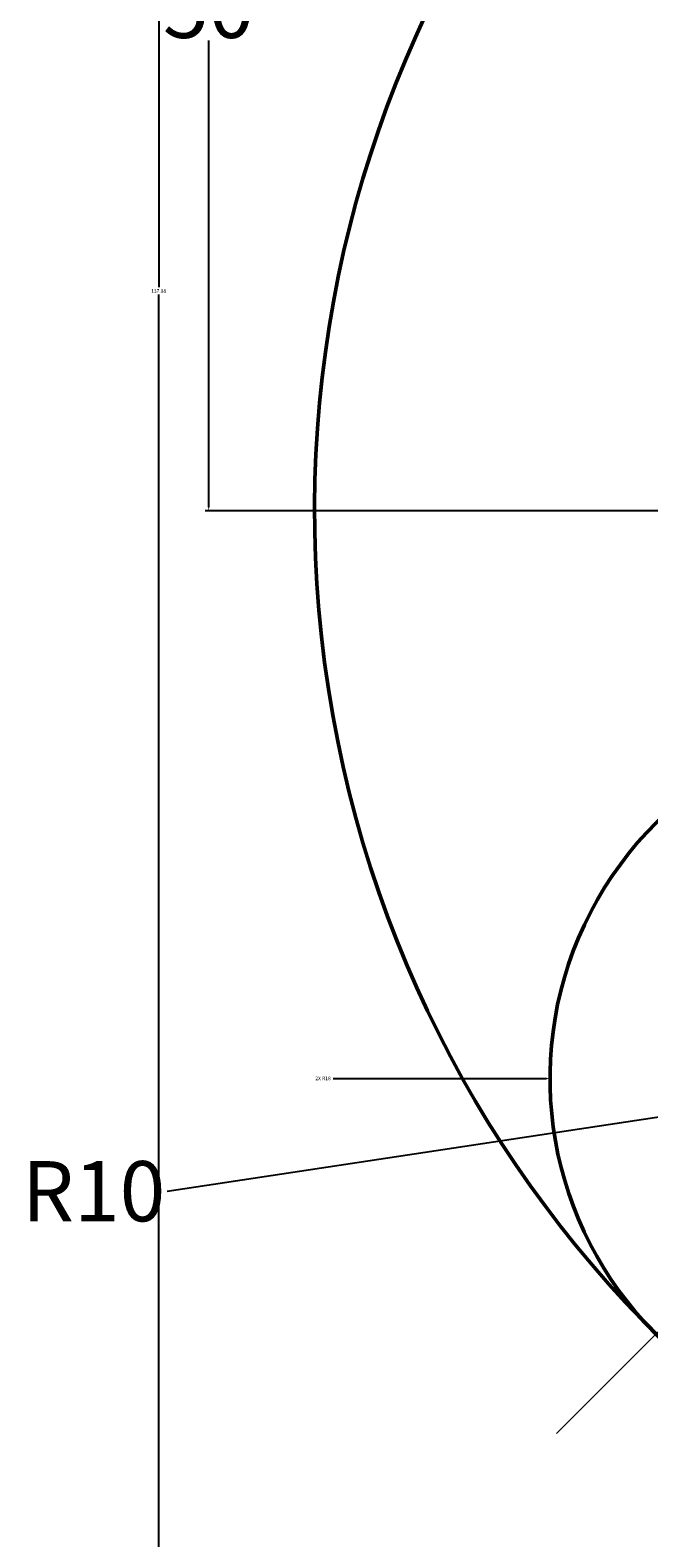
# Model space of a CAD drawing. Units: millimetres. Extents: x -53 to 92, y -147 to 37.
# Tile 2 of 16: x -53 to -22, y -105 to -30. Entities that reach past the tile are written whole.
import ezdxf

# ---------------------------------------------------------------- set-up
doc = ezdxf.new("R2010")
doc.units = ezdxf.units.MM
doc.header["$MEASUREMENT"] = 0
doc.linetypes.add('CENTER', pattern=[50.8, 31.75, -6.35, 6.35, -6.35])
for name, color, linetype, lineweight in [('M-CNTR', 4, 'CENTER', 18), ('M-DIMS', 2, 'Continuous', 25), ('M-OUTL', 7, 'Continuous', 50)]:
    doc.layers.add(name, color=color, linetype=linetype, lineweight=lineweight)
doc.styles.get("Standard").update_dxf_attribs({"font": 'arial.ttf'})
doc.dimstyles.get("Standard").update_dxf_attribs({"dimtxt": 0.18, "dimasz": 0.18, "dimexe": 0.18, "dimexo": 0.0625, "dimgap": 0.09, "dimtad": 0, "dimtih": 1, "dimtoh": 1, "dimdec": 4, "dimzin": 0, "dimdsep": 46, "dimtxsty": 'Standard', "dimcen": 0.09, "dimadec": 0, "dimazin": 0, "dimtfac": 1, "dimtdec": 4, "dimtofl": 0, "dimtmove": 0, "dimatfit": 3, "dimfxl": 1, "dimtolj": 1, "dimtzin": 0, "dimarcsym": 0})

# ---------------------------------------------------------------- blocks, each defined once
blk = doc.blocks.new('*D7')
at = {"layer": 'Defpoints', "color": 0, "transparency": 16777216}
for p in [(9.445, -3.88), (-44.321, -53.98), (18.956, -53.98)]:
    blk.add_point(p, dxfattribs=at)
at = {"layer": 'M-DIMS', "color": 0, "lineweight": -2, "transparency": 16777216}
for p, q in [((9.382, -3.88), (-44.501, -3.88)), ((-44.321, -4.06), (-44.321, -27.308)), ((-44.321, -53.8), (-44.321, -30.552)), ((18.894, -53.98), (-44.501, -53.98))]:
    blk.add_line(p, q, dxfattribs=at)
at = {"layer": 'M-DIMS', "color": 0, "transparency": 16777216}
for points in [[(-44.351, -4.06), (-44.291, -4.06), (-44.321, -3.88)], [(-44.351, -53.8), (-44.291, -53.8), (-44.321, -53.98)]]:
    blk.add_solid(points, dxfattribs=at)
at = {"layer": 'M-DIMS', "color": 0, "transparency": 16777216, "insert": (-44.321, -28.93), "char_height": 0.18, "attachment_point": 5}
blk.add_mtext('\\A1;{\\H16.66667x;50}', dxfattribs=at)
blk = doc.blocks.new('*D8')
at = {"layer": 'Defpoints', "color": 0, "transparency": 16777216}
for p in [(-9.328, -82.264), (-19.215, -83.763)]:
    blk.add_point(p, dxfattribs=at)
at = {"layer": 'M-DIMS', "color": 0, "lineweight": -2, "transparency": 16777216}
for p, q in [((-9.418, -82.264), (-9.238, -82.264)), ((-9.328, -82.354), (-9.328, -82.174)), ((-46.381, -87.879), (-19.393, -83.79))]:
    blk.add_line(p, q, dxfattribs=at)
at = {"layer": 'M-DIMS', "color": 0, "transparency": 16777216}
blk.add_solid([(-19.397, -83.76), (-19.388, -83.819), (-19.215, -83.763)], dxfattribs=at)
at = {"layer": 'M-DIMS', "color": 0, "transparency": 16777216, "insert": (-50.05, -87.879), "char_height": 0.18, "attachment_point": 5}
blk.add_mtext('\\A1;{\\H16.66667x;R10}', dxfattribs=at)
blk = doc.blocks.new('*D10')
at = {"layer": 'Defpoints', "color": 0, "transparency": 16777216}
for p in [(64.593, -18.184), (-26.68, -89.776)]:
    blk.add_point(p, dxfattribs=at)
at = {"layer": 'M-DIMS', "color": 0, "lineweight": -2, "transparency": 16777216}
for p, q in [((77.384, -8.151), (64.734, -18.073)), ((77.564, -8.151), (77.384, -8.151)), ((18.866, -53.98), (19.046, -53.98)), ((18.956, -54.07), (18.956, -53.89))]:
    blk.add_line(p, q, dxfattribs=at)
at = {"layer": 'M-DIMS', "color": 0, "transparency": 16777216}
blk.add_solid([(64.716, -18.05), (64.753, -18.097), (64.593, -18.184)], dxfattribs=at)
at = {"layer": 'M-DIMS', "color": 0, "transparency": 16777216, "insert": (82.599, -8.151), "char_height": 0.18, "attachment_point": 5}
blk.add_mtext('\\A1;{\\H16.66667x;%%C116}', dxfattribs=at)
blk = doc.blocks.new('*D17')
at = {"layer": 'Defpoints', "color": 0, "transparency": 16777216}
for p in [(-46.81, 25.909), (28.564, 25.909), (18.165, -111.975)]:
    blk.add_point(p, dxfattribs=at)
at = {"layer": 'M-DIMS', "color": 0, "lineweight": -2, "transparency": 16777216}
for p, q in [((28.502, 25.909), (-46.99, 25.909)), ((-46.81, 25.729), (-46.81, -42.851)), ((-46.81, -111.795), (-46.81, -43.215)), ((18.102, -111.975), (-46.99, -111.975))]:
    blk.add_line(p, q, dxfattribs=at)
at = {"layer": 'M-DIMS', "color": 0, "transparency": 16777216}
for points in [[(-46.84, 25.729), (-46.78, 25.729), (-46.81, 25.909)], [(-46.84, -111.795), (-46.78, -111.795), (-46.81, -111.975)]]:
    blk.add_solid(points, dxfattribs=at)
at = {"layer": 'M-DIMS', "color": 0, "transparency": 16777216, "insert": (-46.81, -43.033), "char_height": 0.18, "attachment_point": 5}
blk.add_mtext('\\A1;137.88', dxfattribs=at)
blk = doc.blocks.new('*D22')
at = {"layer": 'Defpoints', "color": 0, "transparency": 16777216}
for p in [(-27.328, -82.26), (-9.328, -82.264)]:
    blk.add_point(p, dxfattribs=at)
at = {"layer": 'M-DIMS', "color": 0, "lineweight": -2, "transparency": 16777216}
for p, q in [((-38.128, -82.257), (-27.508, -82.26)), ((-9.418, -82.264), (-9.238, -82.264)), ((-9.328, -82.354), (-9.328, -82.174))]:
    blk.add_line(p, q, dxfattribs=at)
at = {"layer": 'M-DIMS', "color": 0, "transparency": 16777216}
blk.add_solid([(-27.508, -82.23), (-27.508, -82.29), (-27.328, -82.26)], dxfattribs=at)
at = {"layer": 'M-DIMS', "color": 0, "transparency": 16777216, "insert": (-38.628, -82.257), "char_height": 0.18, "attachment_point": 5}
blk.add_mtext('\\A1;2X R18', dxfattribs=at)

msp = doc.modelspace()

# ---------------------------------------------------------------- linework, layer by layer
at = {"layer": 'M-CNTR'}
msp.add_line((18.95638, -53.98007), (-27.00556, -99.94201), dxfattribs=at)
at = {"layer": 'M-OUTL'}
for centre, radius, start, end in [((18.95638, -53.98007), 58, 108.3895553, 70.0459142), ((-9.32787, -82.26433), 18, 84.6241225, 224.9999913)]:
    msp.add_arc(centre, radius, start, end, dxfattribs=at)

# ---------------------------------------------------------------- dimensions: what is measured, and where the dimension line sits
at = {"layer": 'M-DIMS'}
dim = msp.add_linear_dim(base=(-46.8103, 25.90924), p1=(18.16452, -111.97467), p2=(28.56407, 25.90924), angle=90, dimstyle='Standard', override={"dimdec": 2, "dimlfac": 1, "dimrnd": 0, "dimzin": 0, "dimdsep": 46, "dimlunit": 2}, dxfattribs=at)
dim.commit()
dim.dimension.update_dxf_attribs({"geometry": '*D17', "text_midpoint": (-46.8103, -43.03271)})
dim = msp.add_linear_dim(base=(-44.32095, -53.98007), p1=(9.44461, -3.87977), p2=(18.95638, -53.98007), angle=90, text='{\\H16.66667x;50}', dimstyle='Standard', override={"dimclrd": 0, "dimclre": 0, "dimclrt": 0}, dxfattribs=at)
dim.commit()
dim.dimension.update_dxf_attribs({"geometry": '*D7', "text_midpoint": (-44.32095, -28.92992)})
dim = msp.add_diameter_dim_2p(p1=(-26.67986, -89.77579), p2=(64.59262, -18.18435), text='{\\H16.66667x;%%C116}', dimstyle='Standard', override={"dimclrd": 0, "dimclre": 0, "dimclrt": 0}, dxfattribs=at)
dim.commit()
dim.dimension.update_dxf_attribs({"geometry": '*D10', "text_midpoint": (82.59889, -8.15132), "dimtype": 163})
for mpoint, text, override, picture, middle in [((-19.215, -83.76259), '{\\H16.66667x;R10}', {"dimclrd": 0, "dimclre": 0, "dimclrt": 0}, '*D8', (-46.38072, -87.8792)), ((-27.32787, -82.26), '2X <>', {"dimdec": 0, "dimlfac": 1, "dimrnd": 0, "dimzin": 0, "dimdsep": 46, "dimlunit": 2}, '*D22', (-38.12787, -82.2574))]:
    dim = msp.add_radius_dim(center=(-9.32787, -82.26433), mpoint=mpoint, text=text, dimstyle='Standard', override=override, dxfattribs=at)
    dim.commit()
    dim.dimension.update_dxf_attribs({"geometry": picture, "text_midpoint": middle, "dimtype": 164})

doc.saveas('drawing.dxf')
